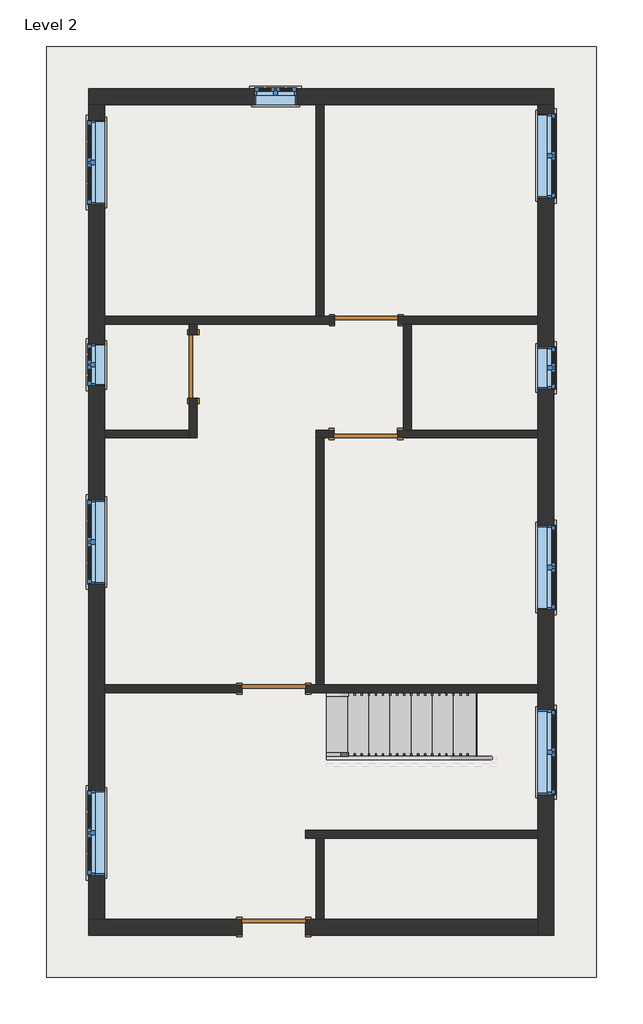
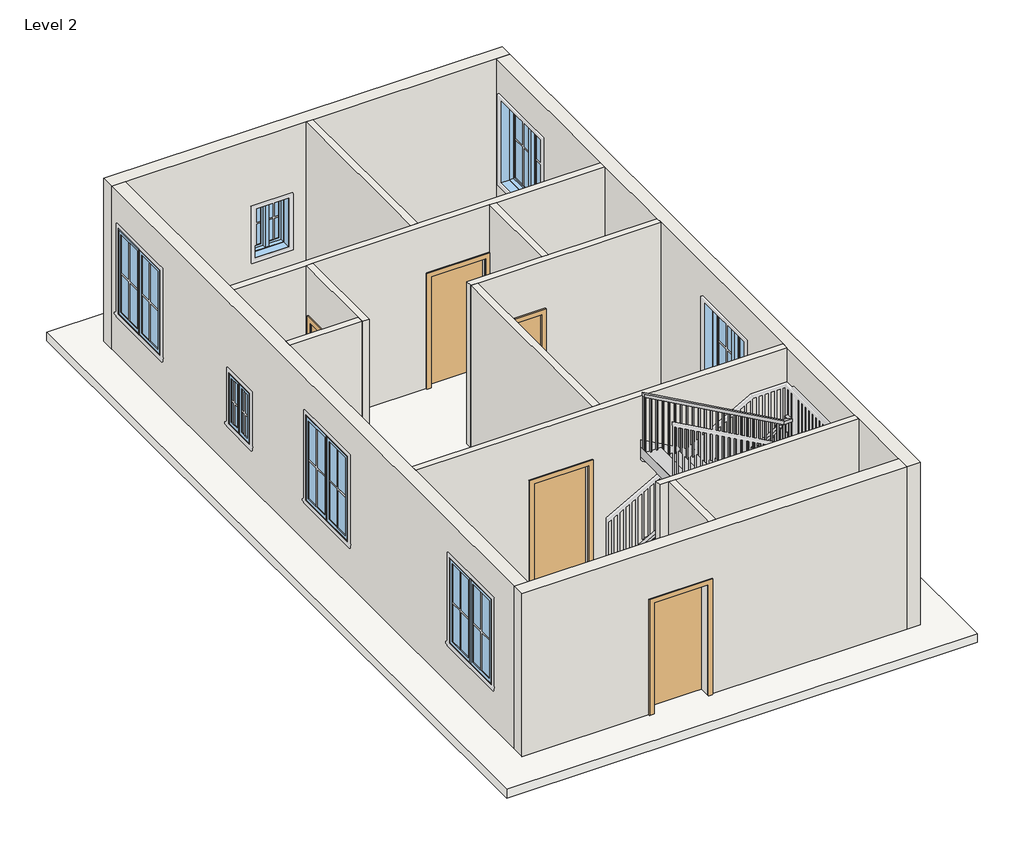
# One storey, part 1 of 2: 14 walls, 9 windows, 5 doors, 1 railing, 1 roof, 1 stair flight.
"""IFC4 building model written with IfcOpenShell, lengths in millimetres."""

from ifc_helpers import new_model, si_unit, frame, origin, place, context, project, spatial, polyline, outline, extrude, faceted_brep, transform, mapped, element, save
from components import door_305aa2a5, door_e5f9f3c4, door_a90ba1ad, stair_flight_0b98486b, window_c417fced, window_8377141f

model = new_model("IFC4")

# Units and contexts
model_context = context("Model", 3, world=origin())
ifc_project = project(units=[si_unit("LENGTHUNIT", "METRE", prefix="MILLI")], contexts=[model_context])

# Site, building, storey
site = spatial("IfcSite", under=ifc_project)
building = spatial("IfcBuilding", under=site)
storey = spatial("IfcBuildingStorey", under=building, Name="Level 2", Elevation=3048.0)

# Doors
placement = place(None, origin())
door_shape = door_305aa2a5(model_context)
element("IfcDoor", 1, ObjectType="Single-Flush : 36\" x 84\"", at=placement, inside=storey, context=model_context, shape_type="MappedRepresentation", body=[
    mapped(door_shape, transform((5270.5, 10636.25, 3048.0), x_axis=(-1.0, 0.0, 0.0), y_axis=(0.0, -1.0, 0.0), z_axis=(0.0, 0.0, 1.0))),
])
door_2_shape = door_e5f9f3c4(model_context)
element("IfcDoor", 2, ObjectType="Single-Flush : 36\" x 84\"", at=placement, inside=storey, context=model_context, shape_type="MappedRepresentation", body=[
    mapped(door_2_shape, transform((2774.95, 9969.5, 3048.0), x_axis=(0.0, 1.0, 0.0), y_axis=(-1.0, 0.0, 0.0), z_axis=(0.0, 0.0, 1.0))),
])
element("IfcDoor", 3, ObjectType="Single-Flush : 36\" x 84\"", at=placement, inside=storey, context=model_context, shape_type="MappedRepresentation", body=[
    mapped(door_2_shape, transform((5264.15, 8997.95, 3048.0), x_axis=(-1.0, 0.0, 0.0), y_axis=(0.0, -1.0, 0.0), z_axis=(0.0, 0.0, 1.0))),
])
element("IfcDoor", 4, ObjectType="Single-Flush : 36\" x 84\"", at=placement, inside=storey, context=model_context, shape_type="MappedRepresentation", body=[
    mapped(door_2_shape, transform((3937.0, 5327.65, 3048.0), x_axis=(1.0, 0.0, 0.0), y_axis=(0.0, 1.0, 0.0), z_axis=(0.0, 0.0, 1.0))),
])
door_3_shape = door_a90ba1ad(model_context)
element("IfcDoor", 5, ObjectType="Single-Flush : 36\" x 84\"", at=placement, inside=storey, context=model_context, shape_type="MappedRepresentation", body=[
    mapped(door_3_shape, transform((3937.0, 1892.3, 3048.0), x_axis=(-1.0, 0.0, 0.0), y_axis=(0.0, -1.0, 0.0), z_axis=(0.0, 0.0, 1.0))),
])

# Railing
element("IfcRailing", 6, ObjectType="Handrail - Rectangular", at=placement, inside=storey, context=model_context, shape_type="SolidModel", body=[
    faceted_brep([(4699.0, 4406.9, 4131.7333333), (4699.0, 4406.9, 4073.620221), (4699.0, 4356.1, 4073.620221), (4699.0, 4356.1, 4131.7333333), (7061.2, 4406.9, 5444.0666667), (7112.0, 4406.9, 5414.1757765), (7112.0, 4356.1, 5414.1757765), (7061.2, 4356.1, 5444.0666667), (7061.2, 4406.9, 5486.4), (7112.0, 4406.9, 5435.6), (7112.0, 4356.1, 5435.6), (7061.2, 4356.1, 5486.4), (7188.2, 4406.9, 5486.4), (7188.2, 4406.9, 5435.6), (7137.4, 4356.1, 5435.6), (7137.4, 4356.1, 5486.4), (7188.2, 4279.9, 5486.4), (7188.2, 4229.1, 5435.6), (7137.4, 4229.1, 5435.6), (7137.4, 4279.9, 5486.4), (7188.2, 4279.9, 5698.0666667), (7188.2, 4229.1, 5647.2666667), (7137.4, 4229.1, 5647.2666667), (7137.4, 4279.9, 5698.0666667), (7188.2, 4152.9, 5698.0666667), (7188.2, 4152.9, 5647.2666667), (7137.4, 4203.7, 5647.2666667), (7137.4, 4203.7, 5698.0666667), (7061.2, 4152.9, 5698.0666667), (7048.0363978, 4152.9, 5647.2666667), (7048.0363978, 4203.7, 5647.2666667), (7061.2, 4203.7, 5698.0666667), (4699.0, 4152.9, 7010.4), (4699.0, 4203.7, 7010.4), (4699.0, 4203.7, 6952.2868876), (4699.0, 4152.9, 6952.2868876)], [[[0, 1, 2, 3]], [[1, 0, 4, 5]], [[2, 1, 5, 6]], [[3, 2, 6, 7]], [[0, 3, 7, 4]], [[5, 4, 8, 9]], [[6, 5, 9, 10]], [[7, 6, 10, 11]], [[4, 7, 11, 8]], [[9, 8, 12, 13]], [[10, 9, 13, 14]], [[11, 10, 14, 15]], [[8, 11, 15, 12]], [[13, 12, 16, 17]], [[14, 13, 17, 18]], [[15, 14, 18, 19]], [[12, 15, 19, 16]], [[17, 16, 20, 21]], [[18, 17, 21, 22]], [[19, 18, 22, 23]], [[16, 19, 23, 20]], [[21, 20, 24, 25]], [[22, 21, 25, 26]], [[23, 22, 26, 27]], [[20, 23, 27, 24]], [[25, 24, 28, 29]], [[26, 25, 29, 30]], [[27, 26, 30, 31]], [[24, 27, 31, 28]], [[32, 33, 34, 35]], [[29, 28, 32, 35]], [[30, 29, 35, 34]], [[31, 30, 34, 33]], [[28, 31, 33, 32]]]),
    extrude(outline(polyline([(6932.8841099, 4733.925), (6943.4674432, 4714.875), (5926.6666667, 4714.875), (5926.6666667, 4733.925), (6932.8841099, 4733.925)])), frame((0.0, 4168.775, 0.0), z_axis=(0.0, 1.0, 0.0), x_axis=(0.0, 0.0, 1.0)), (0.0, 0.0, 1.0), 19.05),
    extrude(outline(polyline([(6876.4396654, 4835.525), (6887.0229988, 4816.475), (5926.6666667, 4816.475), (5926.6666667, 4835.525), (6876.4396654, 4835.525)])), frame((0.0, 4168.775, 0.0), z_axis=(0.0, 1.0, 0.0), x_axis=(0.0, 0.0, 1.0)), (0.0, 0.0, 1.0), 19.05),
    extrude(outline(polyline([(6819.995221, 4937.125), (6830.5785543, 4918.075), (5926.6666667, 4918.075), (5926.6666667, 4937.125), (6819.995221, 4937.125)])), frame((0.0, 4168.775, 0.0), z_axis=(0.0, 1.0, 0.0), x_axis=(0.0, 0.0, 1.0)), (0.0, 0.0, 1.0), 19.05),
    extrude(outline(polyline([(6763.5507765, 5038.725), (6774.1341099, 5019.675), (5757.3333333, 5019.675), (5757.3333333, 5038.725), (6763.5507765, 5038.725)])), frame((0.0, 4168.775, 0.0), z_axis=(0.0, 1.0, 0.0), x_axis=(0.0, 0.0, 1.0)), (0.0, 0.0, 1.0), 19.05),
    extrude(outline(polyline([(6707.1063321, 5140.325), (6717.6896654, 5121.275), (5757.3333333, 5121.275), (5757.3333333, 5140.325), (6707.1063321, 5140.325)])), frame((0.0, 4168.775, 0.0), z_axis=(0.0, 1.0, 0.0), x_axis=(0.0, 0.0, 1.0)), (0.0, 0.0, 1.0), 19.05),
    extrude(outline(polyline([(6650.6618876, 5241.925), (6661.245221, 5222.875), (5757.3333333, 5222.875), (5757.3333333, 5241.925), (6650.6618876, 5241.925)])), frame((0.0, 4168.775, 0.0), z_axis=(0.0, 1.0, 0.0), x_axis=(0.0, 0.0, 1.0)), (0.0, 0.0, 1.0), 19.05),
    extrude(outline(polyline([(6594.2174432, 5343.525), (6604.8007765, 5324.475), (5588.0, 5324.475), (5588.0, 5343.525), (6594.2174432, 5343.525)])), frame((0.0, 4168.775, 0.0), z_axis=(0.0, 1.0, 0.0), x_axis=(0.0, 0.0, 1.0)), (0.0, 0.0, 1.0), 19.05),
    extrude(outline(polyline([(6537.7729988, 5445.125), (6548.3563321, 5426.075), (5588.0, 5426.075), (5588.0, 5445.125), (6537.7729988, 5445.125)])), frame((0.0, 4168.775, 0.0), z_axis=(0.0, 1.0, 0.0), x_axis=(0.0, 0.0, 1.0)), (0.0, 0.0, 1.0), 19.05),
    extrude(outline(polyline([(6481.3285543, 5546.725), (6491.9118876, 5527.675), (5588.0, 5527.675), (5588.0, 5546.725), (6481.3285543, 5546.725)])), frame((0.0, 4168.775, 0.0), z_axis=(0.0, 1.0, 0.0), x_axis=(0.0, 0.0, 1.0)), (0.0, 0.0, 1.0), 19.05),
    extrude(outline(polyline([(6424.8841099, 5648.325), (6435.4674432, 5629.275), (5418.6666667, 5629.275), (5418.6666667, 5648.325), (6424.8841099, 5648.325)])), frame((0.0, 4168.775, 0.0), z_axis=(0.0, 1.0, 0.0), x_axis=(0.0, 0.0, 1.0)), (0.0, 0.0, 1.0), 19.05),
    extrude(outline(polyline([(6368.4396654, 5749.925), (6379.0229988, 5730.875), (5418.6666667, 5730.875), (5418.6666667, 5749.925), (6368.4396654, 5749.925)])), frame((0.0, 4168.775, 0.0), z_axis=(0.0, 1.0, 0.0), x_axis=(0.0, 0.0, 1.0)), (0.0, 0.0, 1.0), 19.05),
    extrude(outline(polyline([(6311.995221, 5851.525), (6322.5785543, 5832.475), (5418.6666667, 5832.475), (5418.6666667, 5851.525), (6311.995221, 5851.525)])), frame((0.0, 4168.775, 0.0), z_axis=(0.0, 1.0, 0.0), x_axis=(0.0, 0.0, 1.0)), (0.0, 0.0, 1.0), 19.05),
    extrude(outline(polyline([(6255.5507765, 5953.125), (6266.1341099, 5934.075), (5249.3333333, 5934.075), (5249.3333333, 5953.125), (6255.5507765, 5953.125)])), frame((0.0, 4168.775, 0.0), z_axis=(0.0, 1.0, 0.0), x_axis=(0.0, 0.0, 1.0)), (0.0, 0.0, 1.0), 19.05),
    extrude(outline(polyline([(6199.1063321, 6054.725), (6209.6896654, 6035.675), (5249.3333333, 6035.675), (5249.3333333, 6054.725), (6199.1063321, 6054.725)])), frame((0.0, 4168.775, 0.0), z_axis=(0.0, 1.0, 0.0), x_axis=(0.0, 0.0, 1.0)), (0.0, 0.0, 1.0), 19.05),
    extrude(outline(polyline([(6142.6618876, 6156.325), (6153.245221, 6137.275), (5249.3333333, 6137.275), (5249.3333333, 6156.325), (6142.6618876, 6156.325)])), frame((0.0, 4168.775, 0.0), z_axis=(0.0, 1.0, 0.0), x_axis=(0.0, 0.0, 1.0)), (0.0, 0.0, 1.0), 19.05),
    extrude(outline(polyline([(6086.2174432, 6257.925), (6096.8007765, 6238.875), (5080.0, 6238.875), (5080.0, 6257.925), (6086.2174432, 6257.925)])), frame((0.0, 4168.775, 0.0), z_axis=(0.0, 1.0, 0.0), x_axis=(0.0, 0.0, 1.0)), (0.0, 0.0, 1.0), 19.05),
    extrude(outline(polyline([(6029.7729988, 6359.525), (6040.3563321, 6340.475), (5080.0, 6340.475), (5080.0, 6359.525), (6029.7729988, 6359.525)])), frame((0.0, 4168.775, 0.0), z_axis=(0.0, 1.0, 0.0), x_axis=(0.0, 0.0, 1.0)), (0.0, 0.0, 1.0), 19.05),
    extrude(outline(polyline([(5973.3285543, 6461.125), (5983.9118876, 6442.075), (5080.0, 6442.075), (5080.0, 6461.125), (5973.3285543, 6461.125)])), frame((0.0, 4168.775, 0.0), z_axis=(0.0, 1.0, 0.0), x_axis=(0.0, 0.0, 1.0)), (0.0, 0.0, 1.0), 19.05),
    extrude(outline(polyline([(5916.8841099, 6562.725), (5927.4674432, 6543.675), (4910.6666667, 6543.675), (4910.6666667, 6562.725), (5916.8841099, 6562.725)])), frame((0.0, 4168.775, 0.0), z_axis=(0.0, 1.0, 0.0), x_axis=(0.0, 0.0, 1.0)), (0.0, 0.0, 1.0), 19.05),
    extrude(outline(polyline([(5860.4396654, 6664.325), (5871.0229988, 6645.275), (4910.6666667, 6645.275), (4910.6666667, 6664.325), (5860.4396654, 6664.325)])), frame((0.0, 4168.775, 0.0), z_axis=(0.0, 1.0, 0.0), x_axis=(0.0, 0.0, 1.0)), (0.0, 0.0, 1.0), 19.05),
    extrude(outline(polyline([(5803.995221, 6765.925), (5814.5785543, 6746.875), (4910.6666667, 6746.875), (4910.6666667, 6765.925), (5803.995221, 6765.925)])), frame((0.0, 4168.775, 0.0), z_axis=(0.0, 1.0, 0.0), x_axis=(0.0, 0.0, 1.0)), (0.0, 0.0, 1.0), 19.05),
    extrude(outline(polyline([(5747.5507765, 6867.525), (5758.1341099, 6848.475), (4741.3333333, 6848.475), (4741.3333333, 6867.525), (5747.5507765, 6867.525)])), frame((0.0, 4168.775, 0.0), z_axis=(0.0, 1.0, 0.0), x_axis=(0.0, 0.0, 1.0)), (0.0, 0.0, 1.0), 19.05),
    extrude(outline(polyline([(5691.1063321, 6969.125), (5701.6896654, 6950.075), (4741.3333333, 6950.075), (4741.3333333, 6969.125), (5691.1063321, 6969.125)])), frame((0.0, 4168.775, 0.0), z_axis=(0.0, 1.0, 0.0), x_axis=(0.0, 0.0, 1.0)), (0.0, 0.0, 1.0), 19.05),
    extrude(outline(polyline([(5634.6618876, 7070.725), (5645.245221, 7051.675), (4741.3333333, 7051.675), (4741.3333333, 7070.725), (5634.6618876, 7070.725)])), frame((0.0, 4168.775, 0.0), z_axis=(0.0, 1.0, 0.0), x_axis=(0.0, 0.0, 1.0)), (0.0, 0.0, 1.0), 19.05),
    extrude(outline(polyline([(7153.275, 4289.425), (7172.325, 4289.425), (7172.325, 4270.375), (7153.275, 4270.375), (7153.275, 4289.425)])), frame((0.0, 0.0, 4572.0), z_axis=(0.0, 0.0, 1.0), x_axis=(1.0, 0.0, 0.0)), (0.0, 0.0, 1.0), 863.6),
    extrude(outline(polyline([(7127.875, 4371.975), (7127.875, 4391.025), (7146.925, 4391.025), (7146.925, 4371.975), (7127.875, 4371.975)])), frame((0.0, 0.0, 4572.0), z_axis=(0.0, 0.0, 1.0), x_axis=(1.0, 0.0, 0.0)), (0.0, 0.0, 1.0), 863.6),
    extrude(outline(polyline([(5377.1341099, 7045.325), (5366.5507765, 7026.275), (4402.6666667, 7026.275), (4402.6666667, 7045.325), (5377.1341099, 7045.325)])), frame((0.0, 4371.975, 0.0), z_axis=(0.0, 1.0, 0.0), x_axis=(0.0, 0.0, 1.0)), (0.0, 0.0, 1.0), 19.05),
    extrude(outline(polyline([(5320.6896654, 6943.725), (5310.1063321, 6924.675), (4402.6666667, 6924.675), (4402.6666667, 6943.725), (5320.6896654, 6943.725)])), frame((0.0, 4371.975, 0.0), z_axis=(0.0, 1.0, 0.0), x_axis=(0.0, 0.0, 1.0)), (0.0, 0.0, 1.0), 19.05),
    extrude(outline(polyline([(5264.245221, 6842.125), (5253.6618876, 6823.075), (4402.6666667, 6823.075), (4402.6666667, 6842.125), (5264.245221, 6842.125)])), frame((0.0, 4371.975, 0.0), z_axis=(0.0, 1.0, 0.0), x_axis=(0.0, 0.0, 1.0)), (0.0, 0.0, 1.0), 19.05),
    extrude(outline(polyline([(5207.8007765, 6740.525), (5197.2174432, 6721.475), (4233.3333333, 6721.475), (4233.3333333, 6740.525), (5207.8007765, 6740.525)])), frame((0.0, 4371.975, 0.0), z_axis=(0.0, 1.0, 0.0), x_axis=(0.0, 0.0, 1.0)), (0.0, 0.0, 1.0), 19.05),
    extrude(outline(polyline([(5151.3563321, 6638.925), (5140.7729988, 6619.875), (4233.3333333, 6619.875), (4233.3333333, 6638.925), (5151.3563321, 6638.925)])), frame((0.0, 4371.975, 0.0), z_axis=(0.0, 1.0, 0.0), x_axis=(0.0, 0.0, 1.0)), (0.0, 0.0, 1.0), 19.05),
    extrude(outline(polyline([(5094.9118876, 6537.325), (5084.3285543, 6518.275), (4233.3333333, 6518.275), (4233.3333333, 6537.325), (5094.9118876, 6537.325)])), frame((0.0, 4371.975, 0.0), z_axis=(0.0, 1.0, 0.0), x_axis=(0.0, 0.0, 1.0)), (0.0, 0.0, 1.0), 19.05),
    extrude(outline(polyline([(5038.4674432, 6435.725), (5027.8841099, 6416.675), (4064.0, 6416.675), (4064.0, 6435.725), (5038.4674432, 6435.725)])), frame((0.0, 4371.975, 0.0), z_axis=(0.0, 1.0, 0.0), x_axis=(0.0, 0.0, 1.0)), (0.0, 0.0, 1.0), 19.05),
    extrude(outline(polyline([(4982.0229988, 6334.125), (4971.4396654, 6315.075), (4064.0, 6315.075), (4064.0, 6334.125), (4982.0229988, 6334.125)])), frame((0.0, 4371.975, 0.0), z_axis=(0.0, 1.0, 0.0), x_axis=(0.0, 0.0, 1.0)), (0.0, 0.0, 1.0), 19.05),
    extrude(outline(polyline([(4925.5785543, 6232.525), (4914.995221, 6213.475), (4064.0, 6213.475), (4064.0, 6232.525), (4925.5785543, 6232.525)])), frame((0.0, 4371.975, 0.0), z_axis=(0.0, 1.0, 0.0), x_axis=(0.0, 0.0, 1.0)), (0.0, 0.0, 1.0), 19.05),
    extrude(outline(polyline([(4869.1341099, 6130.925), (4858.5507765, 6111.875), (3894.6666667, 6111.875), (3894.6666667, 6130.925), (4869.1341099, 6130.925)])), frame((0.0, 4371.975, 0.0), z_axis=(0.0, 1.0, 0.0), x_axis=(0.0, 0.0, 1.0)), (0.0, 0.0, 1.0), 19.05),
    extrude(outline(polyline([(4812.6896654, 6029.325), (4802.1063321, 6010.275), (3894.6666667, 6010.275), (3894.6666667, 6029.325), (4812.6896654, 6029.325)])), frame((0.0, 4371.975, 0.0), z_axis=(0.0, 1.0, 0.0), x_axis=(0.0, 0.0, 1.0)), (0.0, 0.0, 1.0), 19.05),
    extrude(outline(polyline([(4756.245221, 5927.725), (4745.6618876, 5908.675), (3894.6666667, 5908.675), (3894.6666667, 5927.725), (4756.245221, 5927.725)])), frame((0.0, 4371.975, 0.0), z_axis=(0.0, 1.0, 0.0), x_axis=(0.0, 0.0, 1.0)), (0.0, 0.0, 1.0), 19.05),
    extrude(outline(polyline([(4699.8007765, 5826.125), (4689.2174432, 5807.075), (3725.3333333, 5807.075), (3725.3333333, 5826.125), (4699.8007765, 5826.125)])), frame((0.0, 4371.975, 0.0), z_axis=(0.0, 1.0, 0.0), x_axis=(0.0, 0.0, 1.0)), (0.0, 0.0, 1.0), 19.05),
    extrude(outline(polyline([(4643.3563321, 5724.525), (4632.7729988, 5705.475), (3725.3333333, 5705.475), (3725.3333333, 5724.525), (4643.3563321, 5724.525)])), frame((0.0, 4371.975, 0.0), z_axis=(0.0, 1.0, 0.0), x_axis=(0.0, 0.0, 1.0)), (0.0, 0.0, 1.0), 19.05),
    extrude(outline(polyline([(4586.9118876, 5622.925), (4576.3285543, 5603.875), (3725.3333333, 5603.875), (3725.3333333, 5622.925), (4586.9118876, 5622.925)])), frame((0.0, 4371.975, 0.0), z_axis=(0.0, 1.0, 0.0), x_axis=(0.0, 0.0, 1.0)), (0.0, 0.0, 1.0), 19.05),
    extrude(outline(polyline([(4530.4674432, 5521.325), (4519.8841099, 5502.275), (3556.0, 5502.275), (3556.0, 5521.325), (4530.4674432, 5521.325)])), frame((0.0, 4371.975, 0.0), z_axis=(0.0, 1.0, 0.0), x_axis=(0.0, 0.0, 1.0)), (0.0, 0.0, 1.0), 19.05),
    extrude(outline(polyline([(4474.0229988, 5419.725), (4463.4396654, 5400.675), (3556.0, 5400.675), (3556.0, 5419.725), (4474.0229988, 5419.725)])), frame((0.0, 4371.975, 0.0), z_axis=(0.0, 1.0, 0.0), x_axis=(0.0, 0.0, 1.0)), (0.0, 0.0, 1.0), 19.05),
    extrude(outline(polyline([(4417.5785543, 5318.125), (4406.995221, 5299.075), (3556.0, 5299.075), (3556.0, 5318.125), (4417.5785543, 5318.125)])), frame((0.0, 4371.975, 0.0), z_axis=(0.0, 1.0, 0.0), x_axis=(0.0, 0.0, 1.0)), (0.0, 0.0, 1.0), 19.05),
    extrude(outline(polyline([(4361.1341099, 5216.525), (4350.5507765, 5197.475), (3386.6666667, 5197.475), (3386.6666667, 5216.525), (4361.1341099, 5216.525)])), frame((0.0, 4371.975, 0.0), z_axis=(0.0, 1.0, 0.0), x_axis=(0.0, 0.0, 1.0)), (0.0, 0.0, 1.0), 19.05),
    extrude(outline(polyline([(4304.6896654, 5114.925), (4294.1063321, 5095.875), (3386.6666667, 5095.875), (3386.6666667, 5114.925), (4304.6896654, 5114.925)])), frame((0.0, 4371.975, 0.0), z_axis=(0.0, 1.0, 0.0), x_axis=(0.0, 0.0, 1.0)), (0.0, 0.0, 1.0), 19.05),
    extrude(outline(polyline([(4248.245221, 5013.325), (4237.6618876, 4994.275), (3386.6666667, 4994.275), (3386.6666667, 5013.325), (4248.245221, 5013.325)])), frame((0.0, 4371.975, 0.0), z_axis=(0.0, 1.0, 0.0), x_axis=(0.0, 0.0, 1.0)), (0.0, 0.0, 1.0), 19.05),
    extrude(outline(polyline([(4191.8007765, 4911.725), (4181.2174432, 4892.675), (3217.3333333, 4892.675), (3217.3333333, 4911.725), (4191.8007765, 4911.725)])), frame((0.0, 4371.975, 0.0), z_axis=(0.0, 1.0, 0.0), x_axis=(0.0, 0.0, 1.0)), (0.0, 0.0, 1.0), 19.05),
    extrude(outline(polyline([(4135.3563321, 4810.125), (4124.7729988, 4791.075), (3217.3333333, 4791.075), (3217.3333333, 4810.125), (4135.3563321, 4810.125)])), frame((0.0, 4371.975, 0.0), z_axis=(0.0, 1.0, 0.0), x_axis=(0.0, 0.0, 1.0)), (0.0, 0.0, 1.0), 19.05),
    extrude(outline(polyline([(7153.275, 4187.825), (7172.325, 4187.825), (7172.325, 4168.775), (7153.275, 4168.775), (7153.275, 4187.825)])), frame((0.0, 0.0, 4572.0), z_axis=(0.0, 0.0, 1.0), x_axis=(1.0, 0.0, 0.0)), (0.0, 0.0, 1.0), 1075.2666667),
    extrude(outline(polyline([(7153.275, 4371.975), (7153.275, 4391.025), (7172.325, 4391.025), (7172.325, 4371.975), (7153.275, 4371.975)])), frame((0.0, 0.0, 4572.0), z_axis=(0.0, 0.0, 1.0), x_axis=(1.0, 0.0, 0.0)), (0.0, 0.0, 1.0), 863.6),
    extrude(outline(polyline([(6941.7035543, 4718.05), (6952.2868876, 4699.0), (5926.6666667, 4699.0), (5926.6666667, 4718.05), (6941.7035543, 4718.05)])), frame((0.0, 4168.775, 0.0), z_axis=(0.0, 1.0, 0.0), x_axis=(0.0, 0.0, 1.0)), (0.0, 0.0, 1.0), 19.05),
    extrude(outline(polyline([(4084.2035543, 4718.05), (4073.620221, 4699.0), (3217.3333333, 4699.0), (3217.3333333, 4718.05), (4084.2035543, 4718.05)])), frame((0.0, 4371.975, 0.0), z_axis=(0.0, 1.0, 0.0), x_axis=(0.0, 0.0, 1.0)), (0.0, 0.0, 1.0), 19.05),
])

# Roof
element("IfcRoof", 7, ObjectType="Generic - 12\"", at=placement, inside=storey, context=model_context, shape_type="SweptSolid", body=[
    extrude(outline(polyline([(660.4, 14579.6), (8585.2, 14579.6), (8585.2, 1168.4), (660.4, 1168.4), (660.4, 14579.6)])), frame((0.0, 0.0, 3048.0), z_axis=(0.0, 0.0, 1.0), x_axis=(1.0, 0.0, 0.0)), (0.0, 0.0, 1.0), 152.4),
])

# Stair flight
stair_flight_shape = stair_flight_0b98486b(model_context)
element("IfcStairFlight", 8, ObjectType="2\" Tread 1\" Nosing 1/4\" Riser", at=placement, inside=storey, context=model_context, shape_type="MappedRepresentation", body=[
    mapped(stair_flight_shape, transform((0.0, 0.0, 0.0), x_axis=(1.0, 0.0, 0.0), y_axis=(0.0, 1.0, 0.0), z_axis=(0.0, 0.0, 1.0))),
])

# Walls
element("IfcWall", 9, ObjectType="Generic - 5\"", at=placement, inside=storey, context=model_context, shape_type="SweptSolid", body=[
    extrude(outline(polyline([(4546.6, 10693.4), (4546.6, 13741.4), (4660.9, 13741.4), (4660.9, 10693.4), (4546.6, 10693.4)])), frame((0.0, 0.0, 3048.0), z_axis=(0.0, 0.0, 1.0), x_axis=(1.0, 0.0, 0.0)), (0.0, 0.0, 1.0), 3048.0),
])
element("IfcWall", 10, ObjectType="Generic - 5\"", at=placement, inside=storey, context=model_context, shape_type="Brep", body=[
    faceted_brep([(1498.6, 10579.1, 3048.0), (2717.8, 10579.1, 3048.0), (2832.1, 10579.1, 3048.0), (4813.3, 10579.1, 3048.0), (4813.3, 10579.1, 5181.6), (5727.7, 10579.1, 5181.6), (5727.7, 10579.1, 3048.0), (5803.9, 10579.1, 3048.0), (5918.2, 10579.1, 3048.0), (7747.0, 10579.1, 3048.0), (7747.0, 10579.1, 6096.0), (5918.2, 10579.1, 6096.0), (5803.9, 10579.1, 6096.0), (2832.1, 10579.1, 6096.0), (2717.8, 10579.1, 6096.0), (1498.6, 10579.1, 6096.0), (4813.3, 10693.4, 5181.6), (4813.3, 10693.4, 3048.0), (4660.9, 10693.4, 3048.0), (4546.6, 10693.4, 3048.0), (1498.6, 10693.4, 3048.0), (1498.6, 10693.4, 6096.0), (4546.6, 10693.4, 6096.0), (4660.9, 10693.4, 6096.0), (7747.0, 10693.4, 6096.0), (7747.0, 10693.4, 3048.0), (5727.7, 10693.4, 3048.0), (5727.7, 10693.4, 5181.6)], [[[0, 1, 2, 3, 4, 5, 6, 7, 8, 9, 10, 11, 12, 13, 14, 15]], [[16, 17, 18, 19, 20, 21, 22, 23, 24, 25, 26, 27]], [[26, 25, 9, 8, 7, 6]], [[20, 19, 18, 17, 3, 2, 1, 0]], [[15, 14, 13, 12, 11, 10, 24, 23, 22, 21]], [[10, 9, 25, 24]], [[0, 15, 21, 20]], [[4, 3, 17, 16]], [[5, 4, 16, 27]], [[6, 5, 27, 26]]]),
])
element("IfcWall", 11, ObjectType="Generic - 5\"", at=placement, inside=storey, context=model_context, shape_type="Brep", body=[
    faceted_brep([(2717.8, 10579.1, 3048.0), (2717.8, 10426.7, 3048.0), (2717.8, 10426.7, 5181.6), (2717.8, 9512.3, 5181.6), (2717.8, 9512.3, 3048.0), (2717.8, 9055.1, 3048.0), (2717.8, 8940.8, 3048.0), (2717.8, 8940.8, 6096.0), (2717.8, 9055.1, 6096.0), (2717.8, 10579.1, 6096.0), (2832.1, 10426.7, 5181.6), (2832.1, 10426.7, 3048.0), (2832.1, 10579.1, 3048.0), (2832.1, 10579.1, 6096.0), (2832.1, 8940.8, 6096.0), (2832.1, 8940.8, 3048.0), (2832.1, 9512.3, 3048.0), (2832.1, 9512.3, 5181.6)], [[[0, 1, 2, 3, 4, 5, 6, 7, 8, 9]], [[10, 11, 12, 13, 14, 15, 16, 17]], [[16, 15, 6, 5, 4]], [[12, 11, 1, 0]], [[9, 8, 7, 14, 13]], [[0, 9, 13, 12]], [[7, 6, 15, 14]], [[2, 1, 11, 10]], [[3, 2, 10, 17]], [[4, 3, 17, 16]]]),
])
element("IfcWall", 12, ObjectType="Generic - 5\"", at=placement, inside=storey, context=model_context, shape_type="SweptSolid", body=[
    extrude(outline(polyline([(2717.8, 8940.8), (1498.6, 8940.8), (1498.6, 9055.1), (2717.8, 9055.1), (2717.8, 8940.8)])), frame((0.0, 0.0, 3048.0), z_axis=(0.0, 0.0, 1.0), x_axis=(1.0, 0.0, 0.0)), (0.0, 0.0, 1.0), 3048.0),
])
element("IfcWall", 13, ObjectType="Generic - 5\"", at=placement, inside=storey, context=model_context, shape_type="SweptSolid", body=[
    extrude(outline(polyline([(5803.9, 9055.1), (5803.9, 10579.1), (5918.2, 10579.1), (5918.2, 9055.1), (5803.9, 9055.1)])), frame((0.0, 0.0, 3048.0), z_axis=(0.0, 0.0, 1.0), x_axis=(1.0, 0.0, 0.0)), (0.0, 0.0, 1.0), 3048.0),
])
element("IfcWall", 14, ObjectType="Generic - 5\"", at=placement, inside=storey, context=model_context, shape_type="Brep", body=[
    faceted_brep([(4806.95, 9055.1, 5181.6), (4806.95, 9055.1, 3048.0), (4546.6, 9055.1, 3048.0), (4546.6, 9055.1, 6096.0), (5803.9, 9055.1, 6096.0), (5918.2, 9055.1, 6096.0), (7747.0, 9055.1, 6096.0), (7747.0, 9055.1, 3048.0), (5918.2, 9055.1, 3048.0), (5803.9, 9055.1, 3048.0), (5721.35, 9055.1, 3048.0), (5721.35, 9055.1, 5181.6), (4546.6, 8940.8, 3048.0), (4660.9, 8940.8, 3048.0), (4806.95, 8940.8, 3048.0), (4806.95, 8940.8, 5181.6), (5721.35, 8940.8, 5181.6), (5721.35, 8940.8, 3048.0), (7747.0, 8940.8, 3048.0), (7747.0, 8940.8, 6096.0), (4660.9, 8940.8, 6096.0), (4546.6, 8940.8, 6096.0)], [[[0, 1, 2, 3, 4, 5, 6, 7, 8, 9, 10, 11]], [[12, 13, 14, 15, 16, 17, 18, 19, 20, 21]], [[2, 1, 14, 13, 12]], [[10, 9, 8, 7, 18, 17]], [[6, 5, 4, 3, 21, 20, 19]], [[7, 6, 19, 18]], [[3, 2, 12, 21]], [[15, 14, 1, 0]], [[16, 15, 0, 11]], [[17, 16, 11, 10]]]),
])
element("IfcWall", 15, ObjectType="Generic - 5\"", at=placement, inside=storey, context=model_context, shape_type="Brep", body=[
    faceted_brep([(4394.2, 5270.5, 5181.6), (4394.2, 5270.5, 3048.0), (7747.0, 5270.5, 3048.0), (7747.0, 5270.5, 6096.0), (1498.6, 5270.5, 6096.0), (1498.6, 5270.5, 3048.0), (3479.8, 5270.5, 3048.0), (3479.8, 5270.5, 5181.6), (7747.0, 5384.8, 3048.0), (4660.9, 5384.8, 3048.0), (4546.6, 5384.8, 3048.0), (4394.2, 5384.8, 3048.0), (4394.2, 5384.8, 5181.6), (3479.8, 5384.8, 5181.6), (3479.8, 5384.8, 3048.0), (1498.6, 5384.8, 3048.0), (1498.6, 5384.8, 6096.0), (4546.6, 5384.8, 6096.0), (4660.9, 5384.8, 6096.0), (7747.0, 5384.8, 6096.0)], [[[0, 1, 2, 3, 4, 5, 6, 7]], [[8, 9, 10, 11, 12, 13, 14, 15, 16, 17, 18, 19]], [[6, 5, 15, 14]], [[2, 1, 11, 10, 9, 8]], [[4, 3, 19, 18, 17, 16]], [[3, 2, 8, 19]], [[5, 4, 16, 15]], [[12, 11, 1, 0]], [[13, 12, 0, 7]], [[14, 13, 7, 6]]]),
])
element("IfcWall", 16, ObjectType="Generic - 5\"", at=placement, inside=storey, context=model_context, shape_type="SweptSolid", body=[
    extrude(outline(polyline([(4660.9, 8940.8), (4660.9, 5384.8), (4546.6, 5384.8), (4546.6, 8940.8), (4660.9, 8940.8)])), frame((0.0, 0.0, 3048.0), z_axis=(0.0, 0.0, 1.0), x_axis=(1.0, 0.0, 0.0)), (0.0, 0.0, 1.0), 3048.0),
])
element("IfcWall", 17, ObjectType="Generic - 5\"", at=placement, inside=storey, context=model_context, shape_type="SweptSolid", body=[
    extrude(outline(polyline([(4660.9, 3175.0), (4660.9, 2006.6), (4546.6, 2006.6), (4546.6, 3175.0), (4660.9, 3175.0)])), frame((0.0, 0.0, 3048.0), z_axis=(0.0, 0.0, 1.0), x_axis=(1.0, 0.0, 0.0)), (0.0, 0.0, 1.0), 3048.0),
])
element("IfcWall", 18, ObjectType="Generic - 5\"", at=placement, inside=storey, context=model_context, shape_type="Brep", body=[
    faceted_brep([(4394.2, 3175.0, 3048.0), (4546.6, 3175.0, 3048.0), (4660.9, 3175.0, 3048.0), (7747.0, 3175.0, 3048.0), (7747.0, 3175.0, 6096.0), (4660.9, 3175.0, 6096.0), (4546.6, 3175.0, 6096.0), (4394.2, 3175.0, 6096.0), (4394.2, 3289.3, 3048.0), (4394.2, 3289.3, 6096.0), (7747.0, 3289.3, 6096.0), (7747.0, 3289.3, 3048.0)], [[[0, 1, 2, 3, 4, 5, 6, 7]], [[8, 9, 10, 11]], [[3, 2, 1, 0, 8, 11]], [[7, 6, 5, 4, 10, 9]], [[0, 7, 9, 8]], [[4, 3, 11, 10]]]),
])
element("IfcWall", 19, ObjectType="Generic - 8\"", at=placement, inside=storey, context=model_context, shape_type="Brep", body=[
    faceted_brep([(1270.0, 13741.4, 3048.0), (1498.6, 13741.4, 3048.0), (4546.6, 13741.4, 3048.0), (4660.9, 13741.4, 3048.0), (7747.0, 13741.4, 3048.0), (7975.6, 13741.4, 3048.0), (7975.6, 13741.4, 6096.0), (7747.0, 13741.4, 6096.0), (4660.9, 13741.4, 6096.0), (4546.6, 13741.4, 6096.0), (1498.6, 13741.4, 6096.0), (1270.0, 13741.4, 6096.0), (4267.2, 13741.4, 4876.8), (4267.2, 13741.4, 3962.4), (3657.6, 13741.4, 3962.4), (3657.6, 13741.4, 4876.8), (1270.0, 13970.0, 3048.0), (1270.0, 13970.0, 6096.0), (7975.6, 13970.0, 6096.0), (7975.6, 13970.0, 3048.0), (4267.2, 13970.0, 4876.8), (3657.6, 13970.0, 4876.8), (3657.6, 13970.0, 3962.4), (4267.2, 13970.0, 3962.4)], [[[0, 1, 2, 3, 4, 5, 6, 7, 8, 9, 10, 11], [12, 13, 14, 15]], [[16, 17, 18, 19], [20, 21, 22, 23]], [[5, 4, 3, 2, 1, 0, 16, 19]], [[11, 10, 9, 8, 7, 6, 18, 17]], [[6, 5, 19, 18]], [[0, 11, 17, 16]], [[13, 12, 20, 23]], [[14, 13, 23, 22]], [[15, 14, 22, 21]], [[12, 15, 21, 20]]]),
])
element("IfcWall", 20, ObjectType="Generic - 8\"", at=placement, inside=storey, context=model_context, shape_type="Brep", body=[
    faceted_brep([(7747.0, 13741.4, 3048.0), (7747.0, 10693.4, 3048.0), (7747.0, 10579.1, 3048.0), (7747.0, 9055.1, 3048.0), (7747.0, 8940.8, 3048.0), (7747.0, 5384.8, 3048.0), (7747.0, 5270.5, 3048.0), (7747.0, 3289.3, 3048.0), (7747.0, 3175.0, 3048.0), (7747.0, 2006.6, 3048.0), (7747.0, 1778.0, 3048.0), (7747.0, 1778.0, 6096.0), (7747.0, 2006.6, 6096.0), (7747.0, 3175.0, 6096.0), (7747.0, 3289.3, 6096.0), (7747.0, 5270.5, 6096.0), (7747.0, 5384.8, 6096.0), (7747.0, 8940.8, 6096.0), (7747.0, 9055.1, 6096.0), (7747.0, 10579.1, 6096.0), (7747.0, 10693.4, 6096.0), (7747.0, 13741.4, 6096.0), (7747.0, 12395.2, 5486.4), (7747.0, 12395.2, 3962.4), (7747.0, 13614.4, 3962.4), (7747.0, 13614.4, 5486.4), (7747.0, 6464.3, 5486.4), (7747.0, 6464.3, 3962.4), (7747.0, 7683.5, 3962.4), (7747.0, 7683.5, 5486.4), (7747.0, 9645.65, 4876.8), (7747.0, 9645.65, 3962.4), (7747.0, 10255.25, 3962.4), (7747.0, 10255.25, 4876.8), (7747.0, 3803.65, 5486.4), (7747.0, 3803.65, 3962.4), (7747.0, 5022.85, 3962.4), (7747.0, 5022.85, 5486.4), (7975.6, 13741.4, 3048.0), (7975.6, 13741.4, 6096.0), (7975.6, 1778.0, 6096.0), (7975.6, 1778.0, 3048.0), (7975.6, 12395.2, 5486.4), (7975.6, 13614.4, 5486.4), (7975.6, 13614.4, 3962.4), (7975.6, 12395.2, 3962.4), (7975.6, 6464.3, 5486.4), (7975.6, 7683.5, 5486.4), (7975.6, 7683.5, 3962.4), (7975.6, 6464.3, 3962.4), (7975.6, 9645.65, 4876.8), (7975.6, 10255.25, 4876.8), (7975.6, 10255.25, 3962.4), (7975.6, 9645.65, 3962.4), (7975.6, 3803.65, 5486.4), (7975.6, 5022.85, 5486.4), (7975.6, 5022.85, 3962.4), (7975.6, 3803.65, 3962.4)], [[[0, 1, 2, 3, 4, 5, 6, 7, 8, 9, 10, 11, 12, 13, 14, 15, 16, 17, 18, 19, 20, 21], [22, 23, 24, 25], [26, 27, 28, 29], [30, 31, 32, 33], [34, 35, 36, 37]], [[38, 39, 40, 41], [42, 43, 44, 45], [46, 47, 48, 49], [50, 51, 52, 53], [54, 55, 56, 57]], [[10, 9, 8, 7, 6, 5, 4, 3, 2, 1, 0, 38, 41]], [[21, 20, 19, 18, 17, 16, 15, 14, 13, 12, 11, 40, 39]], [[0, 21, 39, 38]], [[11, 10, 41, 40]], [[23, 22, 42, 45]], [[24, 23, 45, 44]], [[25, 24, 44, 43]], [[22, 25, 43, 42]], [[27, 26, 46, 49]], [[28, 27, 49, 48]], [[29, 28, 48, 47]], [[26, 29, 47, 46]], [[31, 30, 50, 53]], [[32, 31, 53, 52]], [[33, 32, 52, 51]], [[30, 33, 51, 50]], [[35, 34, 54, 57]], [[36, 35, 57, 56]], [[37, 36, 56, 55]], [[34, 37, 55, 54]]]),
])
element("IfcWall", 21, ObjectType="Generic - 8\"", at=placement, inside=storey, context=model_context, shape_type="Brep", body=[
    faceted_brep([(3479.8, 2006.6, 5181.6), (3479.8, 2006.6, 3048.0), (1498.6, 2006.6, 3048.0), (1270.0, 2006.6, 3048.0), (1270.0, 2006.6, 6096.0), (1498.6, 2006.6, 6096.0), (4546.6, 2006.6, 6096.0), (4660.9, 2006.6, 6096.0), (7747.0, 2006.6, 6096.0), (7747.0, 2006.6, 3048.0), (4660.9, 2006.6, 3048.0), (4546.6, 2006.6, 3048.0), (4394.2, 2006.6, 3048.0), (4394.2, 2006.6, 5181.6), (1270.0, 1778.0, 3048.0), (3479.8, 1778.0, 3048.0), (3479.8, 1778.0, 5181.6), (4394.2, 1778.0, 5181.6), (4394.2, 1778.0, 3048.0), (7747.0, 1778.0, 3048.0), (7747.0, 1778.0, 6096.0), (1270.0, 1778.0, 6096.0)], [[[0, 1, 2, 3, 4, 5, 6, 7, 8, 9, 10, 11, 12, 13]], [[14, 15, 16, 17, 18, 19, 20, 21]], [[3, 2, 1, 15, 14]], [[12, 11, 10, 9, 19, 18]], [[8, 7, 6, 5, 4, 21, 20]], [[9, 8, 20, 19]], [[4, 3, 14, 21]], [[16, 15, 1, 0]], [[17, 16, 0, 13]], [[18, 17, 13, 12]]]),
])
element("IfcWall", 22, ObjectType="Generic - 8\"", at=placement, inside=storey, context=model_context, shape_type="Brep", body=[
    faceted_brep([(1498.6, 2006.6, 3048.0), (1498.6, 5270.5, 3048.0), (1498.6, 5384.8, 3048.0), (1498.6, 8940.8, 3048.0), (1498.6, 9055.1, 3048.0), (1498.6, 10579.1, 3048.0), (1498.6, 10693.4, 3048.0), (1498.6, 13741.4, 3048.0), (1498.6, 13741.4, 6096.0), (1498.6, 10693.4, 6096.0), (1498.6, 10579.1, 6096.0), (1498.6, 9055.1, 6096.0), (1498.6, 8940.8, 6096.0), (1498.6, 5384.8, 6096.0), (1498.6, 5270.5, 6096.0), (1498.6, 2006.6, 6096.0), (1498.6, 3860.3039063, 5486.4), (1498.6, 3860.3039063, 3962.4), (1498.6, 2641.1039063, 3962.4), (1498.6, 2641.1039063, 5486.4), (1498.6, 8051.3039062, 5486.4), (1498.6, 8051.3039062, 3962.4), (1498.6, 6832.1039062, 3962.4), (1498.6, 6832.1039062, 5486.4), (1498.6, 13518.6539062, 5486.4), (1498.6, 13518.6539062, 3962.4), (1498.6, 12299.4539062, 3962.4), (1498.6, 12299.4539062, 5486.4), (1498.6, 10299.2039062, 4876.8), (1498.6, 10299.2039062, 3962.4), (1498.6, 9689.6039062, 3962.4), (1498.6, 9689.6039062, 4876.8), (1270.0, 2006.6, 3048.0), (1270.0, 2006.6, 6096.0), (1270.0, 13741.4, 6096.0), (1270.0, 13741.4, 3048.0), (1270.0, 3860.3039063, 5486.4), (1270.0, 2641.1039063, 5486.4), (1270.0, 2641.1039063, 3962.4), (1270.0, 3860.3039063, 3962.4), (1270.0, 8051.3039062, 5486.4), (1270.0, 6832.1039062, 5486.4), (1270.0, 6832.1039062, 3962.4), (1270.0, 8051.3039062, 3962.4), (1270.0, 13518.6539062, 5486.4), (1270.0, 12299.4539062, 5486.4), (1270.0, 12299.4539062, 3962.4), (1270.0, 13518.6539062, 3962.4), (1270.0, 10299.2039062, 4876.8), (1270.0, 9689.6039062, 4876.8), (1270.0, 9689.6039062, 3962.4), (1270.0, 10299.2039062, 3962.4)], [[[0, 1, 2, 3, 4, 5, 6, 7, 8, 9, 10, 11, 12, 13, 14, 15], [16, 17, 18, 19], [20, 21, 22, 23], [24, 25, 26, 27], [28, 29, 30, 31]], [[32, 33, 34, 35], [36, 37, 38, 39], [40, 41, 42, 43], [44, 45, 46, 47], [48, 49, 50, 51]], [[7, 6, 5, 4, 3, 2, 1, 0, 32, 35]], [[15, 14, 13, 12, 11, 10, 9, 8, 34, 33]], [[0, 15, 33, 32]], [[8, 7, 35, 34]], [[17, 16, 36, 39]], [[18, 17, 39, 38]], [[19, 18, 38, 37]], [[16, 19, 37, 36]], [[21, 20, 40, 43]], [[22, 21, 43, 42]], [[23, 22, 42, 41]], [[20, 23, 41, 40]], [[25, 24, 44, 47]], [[26, 25, 47, 46]], [[27, 26, 46, 45]], [[24, 27, 45, 44]], [[29, 28, 48, 51]], [[30, 29, 51, 50]], [[31, 30, 50, 49]], [[28, 31, 49, 48]]]),
])

# Windows
window_shape = window_c417fced(model_context)
element("IfcWindow", 23, ObjectType="Window-Casement-Double : 24\" x 36\"", at=placement, inside=storey, context=model_context, shape_type="MappedRepresentation", body=[
    mapped(window_shape, transform((3962.4, 13855.7, 3048.0), x_axis=(1.0, 0.0, 0.0), y_axis=(0.0, 1.0, 0.0), z_axis=(0.0, 0.0, 1.0))),
])
element("IfcWindow", 24, ObjectType="Window-Casement-Double : 24\" x 36\"", at=placement, inside=storey, context=model_context, shape_type="MappedRepresentation", body=[
    mapped(window_shape, transform((7861.3, 9950.45, 3048.0), x_axis=(0.0, -1.0, 0.0), y_axis=(1.0, 0.0, 0.0), z_axis=(0.0, 0.0, 1.0))),
])
element("IfcWindow", 25, ObjectType="Window-Casement-Double : 24\" x 36\"", at=placement, inside=storey, context=model_context, shape_type="MappedRepresentation", body=[
    mapped(window_shape, transform((1384.3, 9994.4039062, 3048.0), x_axis=(0.0, 1.0, 0.0), y_axis=(-1.0, 0.0, 0.0), z_axis=(0.0, 0.0, 1.0))),
])
window_2_shape = window_8377141f(model_context)
element("IfcWindow", 26, ObjectType="Window-Casement-Double : 48\" x 60\"", at=placement, inside=storey, context=model_context, shape_type="MappedRepresentation", body=[
    mapped(window_2_shape, transform((1384.3, 3250.7039063, 3048.0), x_axis=(0.0, 1.0, 0.0), y_axis=(-1.0, 0.0, 0.0), z_axis=(0.0, 0.0, 1.0))),
])
element("IfcWindow", 27, ObjectType="Window-Casement-Double : 48\" x 60\"", at=placement, inside=storey, context=model_context, shape_type="MappedRepresentation", body=[
    mapped(window_2_shape, transform((1384.3, 7441.7039063, 3048.0), x_axis=(0.0, 1.0, 0.0), y_axis=(-1.0, 0.0, 0.0), z_axis=(0.0, 0.0, 1.0))),
])
element("IfcWindow", 28, ObjectType="Window-Casement-Double : 48\" x 60\"", at=placement, inside=storey, context=model_context, shape_type="MappedRepresentation", body=[
    mapped(window_2_shape, transform((1384.3, 12909.0539063, 3048.0), x_axis=(0.0, 1.0, 0.0), y_axis=(-1.0, 0.0, 0.0), z_axis=(0.0, 0.0, 1.0))),
])
element("IfcWindow", 29, ObjectType="Window-Casement-Double : 48\" x 60\"", at=placement, inside=storey, context=model_context, shape_type="MappedRepresentation", body=[
    mapped(window_2_shape, transform((7861.3, 13004.8, 3048.0), x_axis=(0.0, -1.0, 0.0), y_axis=(1.0, 0.0, 0.0), z_axis=(0.0, 0.0, 1.0))),
])
element("IfcWindow", 30, ObjectType="Window-Casement-Double : 48\" x 60\"", at=placement, inside=storey, context=model_context, shape_type="MappedRepresentation", body=[
    mapped(window_2_shape, transform((7861.3, 7073.9, 3048.0), x_axis=(0.0, -1.0, 0.0), y_axis=(1.0, 0.0, 0.0), z_axis=(0.0, 0.0, 1.0))),
])
element("IfcWindow", 31, ObjectType="Window-Casement-Double : 48\" x 60\"", at=placement, inside=storey, context=model_context, shape_type="MappedRepresentation", body=[
    mapped(window_2_shape, transform((7861.3, 4413.25, 3048.0), x_axis=(0.0, -1.0, 0.0), y_axis=(1.0, 0.0, 0.0), z_axis=(0.0, 0.0, 1.0))),
])

save(model, "model.ifc")

# Revit data of these elements
# Type "Single-Flush : 36\" x 84\""
#   Type Mark = "1"
#   Construction Type Id = "MDOOR"
#   Assembly Code = "C1020"
#   Analytic Construction = "Metal"
#   Thickness = 0' - 2"
#   Heat Transfer Coefficient (U) = 0.651978 BTU/(h·ft²·°F)
#   Height = 7' - 0"
#   Trim Projection Ext = 0' - 1"
#   Trim Projection Int = 0' - 1"
#   Trim Width = 0' - 3"
#   Width = 3' - 0"
#   Define Thermal Properties by = 1
#   Define Thermal Properties by = 1
#   Door Material = Door - Panel
#   Frame Material = Door - Frame
#   Visual Light Transmittance = 0
#   Solar Heat Gain Coefficient = 0
#   Function = (empty or 0)
#   Wall Closure = (empty or 0)
# Type "Handrail - Rectangular"
#   Assembly Code = "C2010400"
#   built-in parameter 1008612 = 0.0416667 (stored number, unit not read)
#   built-in parameter 1008611 = 0.0416667 (stored number, unit not read)
#   built-in parameter 1008609 = 0.333333 (stored number, unit not read)
#   built-in parameter 1008604 = 0.166667 (stored number, unit not read)
#   built-in parameter 1008603 = 0.166667 (stored number, unit not read)
#   Railing Height = 3' - 0"
#   built-in parameter 1008630 = 2
#   built-in parameter 1008610 = 2
#   built-in parameter 1008618 = Baluster - Square : 3/4"
# Type "Generic - 12\""
#   Assembly Code = "B1020"
#   Layers, outside or top first: 0' - 6" no material (function 1)
# Type "Generic - 5\""
#   Assembly Code = "B2010"
#   Layers, outside or top first: 0' - 4 1/2" no material (function 1)
# Type "Generic - 8\""
#   Assembly Code = "B2010"
#   Layers, outside or top first: 0' - 9" no material (function 1)
# Type "Window-Casement-Double : 24\" x 36\""
#   Type Mark = "14"
#   Fire Rating = "0.5h"
#   Assembly Code = "B2020100"
#   Analytic Construction = "Double glazing - domestic"
#   Frame Extension [instance default] = 0' - 0 1/4"
#   Window Inset [instance default] = 0' - 0"
#   Wall Thickness [instance default] = 0' - 6"
#   Interior Wall Closure [instance default] = 0' - 2 1/4"
#   Half Width = 1' - 0"
#   Visual Light Transmittance = 0.81
#   Thermal Resistance (R) = 1.8146 (h·ft²·°F)/BTU
#   Solar Heat Gain Coefficient = 0.76
#   Rough Width = 2' - 0 1/2"
#   Rough Height = 3' - 0 1/2"
#   Height = 3' - 0"
#   Heat Transfer Coefficient (U) = 0.5511 BTU/(h·ft²·°F)
#   Exterior Wall Closure [instance default] = 0' - 1 1/4"
#   Extension Jamb [instance default] = 0' - 2 1/4"
#   Default Sill Height = 3' - 0"
#   Width = 2' - 0"
#   Define Thermal Properties by = 0
#   Muntin Visibility = yes
#   Interior Trim Visibility [instance default] = yes
#   Exterior Trim Visibility [instance default] = yes
#   Extension Jamb Visibility [instance default] = yes
#   Interior Trim Material = Wood - Stained
#   Muntin Pattern = Muntin Pattern_2x2 : Muntin Pattern_2x2
#   Interior Trim = Trim-Window-Interior-Flat : Picture Frame
#   Interior Frame Material = Wood - Stained
#   Glass Panel Material = Glass
#   Exterior Trim Material = Clad - White
#   Exterior Trim = Trim-Window-Exterior-Flat : with Sill
#   Exterior Frame Material = Clad - White
#   Wall Closure = (empty or 0)
# Type "Window-Casement-Double : 48\" x 60\""
#   Type Mark = "17"
#   Fire Rating = "0.5h"
#   Assembly Code = "B2020100"
#   Analytic Construction = "Double glazing - domestic"
#   Frame Extension [instance default] = 0' - 0 1/4"
#   Window Inset [instance default] = 0' - 0"
#   Wall Thickness [instance default] = 0' - 6"
#   Interior Wall Closure [instance default] = 0' - 2 1/4"
#   Half Width = 2' - 0"
#   Visual Light Transmittance = 0.81
#   Thermal Resistance (R) = 1.8146 (h·ft²·°F)/BTU
#   Solar Heat Gain Coefficient = 0.76
#   Rough Width = 4' - 0 1/2"
#   Rough Height = 5' - 0 1/2"
#   Height = 5' - 0"
#   Heat Transfer Coefficient (U) = 0.5511 BTU/(h·ft²·°F)
#   Exterior Wall Closure [instance default] = 0' - 1 1/4"
#   Extension Jamb [instance default] = 0' - 2 1/4"
#   Default Sill Height = 3' - 0"
#   Width = 4' - 0"
#   Define Thermal Properties by = 0
#   Muntin Visibility = yes
#   Interior Trim Visibility [instance default] = yes
#   Exterior Trim Visibility [instance default] = yes
#   Extension Jamb Visibility [instance default] = yes
#   Interior Trim Material = Wood - Stained
#   Muntin Pattern = Muntin Pattern_2x2 : Muntin Pattern_2x2
#   Interior Trim = Trim-Window-Interior-Flat : Picture Frame
#   Interior Frame Material = Wood - Stained
#   Glass Panel Material = Glass
#   Exterior Trim Material = Clad - White
#   Exterior Trim = Trim-Window-Exterior-Flat : with Sill
#   Exterior Frame Material = Clad - White
#   Wall Closure = (empty or 0)
# Elements 1, 2, 3, 4, 5 (IfcDoor, "Single-Flush : 36\" x 84\"")
#   Phase Created = New Construction
#   Materials on its faces: "Door - Frame", "Door - Panel"
# Element 6 (IfcRailing, "Handrail - Rectangular")
#   Phase Created = New Construction
# Element 7 (IfcRoof, "Generic - 12\"")
#   built-in parameter 1001705 = 10.5 (stored number, unit not read)
#   built-in parameter 1001710 = 33615
#   Phase Created = New Construction
#   Materials on its faces: "Textile - Linen, Smooth", "Default Roof"
# Element 8 (IfcStairFlight, "2\" Tread 1\" Nosing 1/4\" Riser")
#   Phase Created = New Construction
# Elements 9, 10, 11, 12, 13, 14, 15, 16, 17, 18 (IfcWall, "Generic - 5\"")
#   Top Offset = 0' - 0"
#   Base Offset = 0' - 0"
#   wall height = 10' - 0"
#   Phase Created = New Construction
#   Base Constraint = Level 2
#   Top Constraint = Level 3
#   Materials on its faces: "Default Wall"
# Elements 19, 20, 21, 22 (IfcWall, "Generic - 8\"")
#   Top Offset = 0' - 0"
#   Base Offset = 0' - 0"
#   Unconnected Height = 10' - 0"
#   wall height = 10' - 0"
#   Phase Created = New Construction
#   Base Constraint = Level 2
#   Materials on its faces: "Default Wall", "Wood - Stained"
# Element 23 (IfcWindow, "Window-Casement-Double : 24\" x 36\"")
#   Mark = "16"
#   Window Inset = 0' - 0"
#   Interior Wall Closure = 0' - 2 1/4"
#   Frame Extension = 0' - 0 1/4"
#   Exterior Wall Closure = 0' - 1 1/4"
#   Interior Trim Visibility = yes
#   Exterior Trim Visibility = yes
#   Phase Created = New Construction
#   Materials on its faces: "Wood - Stained", "Glass", "Clad - White"
# Element 24 (IfcWindow, "Window-Casement-Double : 24\" x 36\"")
#   Mark = "17"
#   Window Inset = 0' - 0"
#   Interior Wall Closure = 0' - 2 1/4"
#   Frame Extension = 0' - 0 1/4"
#   Exterior Wall Closure = 0' - 1 1/4"
#   Interior Trim Visibility = yes
#   Exterior Trim Visibility = yes
#   Phase Created = New Construction
#   Materials on its faces: "Wood - Stained", "Glass", "Clad - White"
# Element 25 (IfcWindow, "Window-Casement-Double : 24\" x 36\"")
#   Mark = "18"
#   Window Inset = 0' - 0"
#   Interior Wall Closure = 0' - 2 1/4"
#   Frame Extension = 0' - 0 1/4"
#   Exterior Wall Closure = 0' - 1 1/4"
#   Interior Trim Visibility = yes
#   Exterior Trim Visibility = yes
#   Phase Created = New Construction
#   Materials on its faces: "Wood - Stained", "Glass", "Clad - White"
# Element 26 (IfcWindow, "Window-Casement-Double : 48\" x 60\"")
#   Mark = "11"
#   Window Inset = 0' - 0"
#   Interior Wall Closure = 0' - 2 1/4"
#   Frame Extension = 0' - 0 1/4"
#   Exterior Wall Closure = 0' - 1 1/4"
#   Interior Trim Visibility = yes
#   Exterior Trim Visibility = yes
#   Phase Created = New Construction
#   Materials on its faces: "Wood - Stained", "Glass", "Clad - White"
# Element 27 (IfcWindow, "Window-Casement-Double : 48\" x 60\"")
#   Mark = "12"
#   Window Inset = 0' - 0"
#   Interior Wall Closure = 0' - 2 1/4"
#   Frame Extension = 0' - 0 1/4"
#   Exterior Wall Closure = 0' - 1 1/4"
#   Interior Trim Visibility = yes
#   Exterior Trim Visibility = yes
#   Phase Created = New Construction
#   Materials on its faces: "Wood - Stained", "Glass", "Clad - White"
# Element 28 (IfcWindow, "Window-Casement-Double : 48\" x 60\"")
#   Mark = "13"
#   Window Inset = 0' - 0"
#   Interior Wall Closure = 0' - 2 1/4"
#   Frame Extension = 0' - 0 1/4"
#   Exterior Wall Closure = 0' - 1 1/4"
#   Interior Trim Visibility = yes
#   Exterior Trim Visibility = yes
#   Phase Created = New Construction
#   Materials on its faces: "Wood - Stained", "Glass", "Clad - White"
# Element 29 (IfcWindow, "Window-Casement-Double : 48\" x 60\"")
#   Mark = "14"
#   Window Inset = 0' - 0"
#   Interior Wall Closure = 0' - 2 1/4"
#   Frame Extension = 0' - 0 1/4"
#   Exterior Wall Closure = 0' - 1 1/4"
#   Interior Trim Visibility = yes
#   Exterior Trim Visibility = yes
#   Phase Created = New Construction
#   Materials on its faces: "Wood - Stained", "Glass", "Clad - White"
# Element 30 (IfcWindow, "Window-Casement-Double : 48\" x 60\"")
#   Mark = "15"
#   Window Inset = 0' - 0"
#   Interior Wall Closure = 0' - 2 1/4"
#   Frame Extension = 0' - 0 1/4"
#   Exterior Wall Closure = 0' - 1 1/4"
#   Interior Trim Visibility = yes
#   Exterior Trim Visibility = yes
#   Phase Created = New Construction
#   Materials on its faces: "Wood - Stained", "Glass", "Clad - White"
# Element 31 (IfcWindow, "Window-Casement-Double : 48\" x 60\"")
#   Mark = "19"
#   Window Inset = 0' - 0"
#   Interior Wall Closure = 0' - 2 1/4"
#   Frame Extension = 0' - 0 1/4"
#   Exterior Wall Closure = 0' - 1 1/4"
#   Interior Trim Visibility = yes
#   Exterior Trim Visibility = yes
#   Phase Created = New Construction
#   Materials on its faces: "Wood - Stained", "Glass", "Clad - White"
# Materials
#   "Door - Panel": class "Wood", colour RGB 210 159 95, transparency 0, Cost = 0
#   "Door - Frame": colour RGB 118 70 51, transparency 0, Cost = 0
#   "Wood - Stained": class "Wood", colour RGB 224 178 126, transparency 0, Cost = 0
#   "Glass": class "Glass", colour RGB 0 128 192, transparency 0.75, Description = "Soda Lime Glass", Cost = 0
#   "Clad - White": class "Wood", colour RGB 242 242 238, transparency 0, Cost = 0
#   "Textile - Linen, Smooth": colour RGB 249 239 230, transparency 0
#   "Default Roof": colour RGB 88 101 114, transparency 0, Cost = 0
#   "Default Wall": colour RGB 128 128 128, transparency 0, Cost = 0
